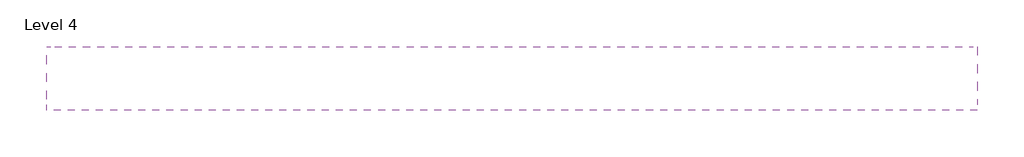
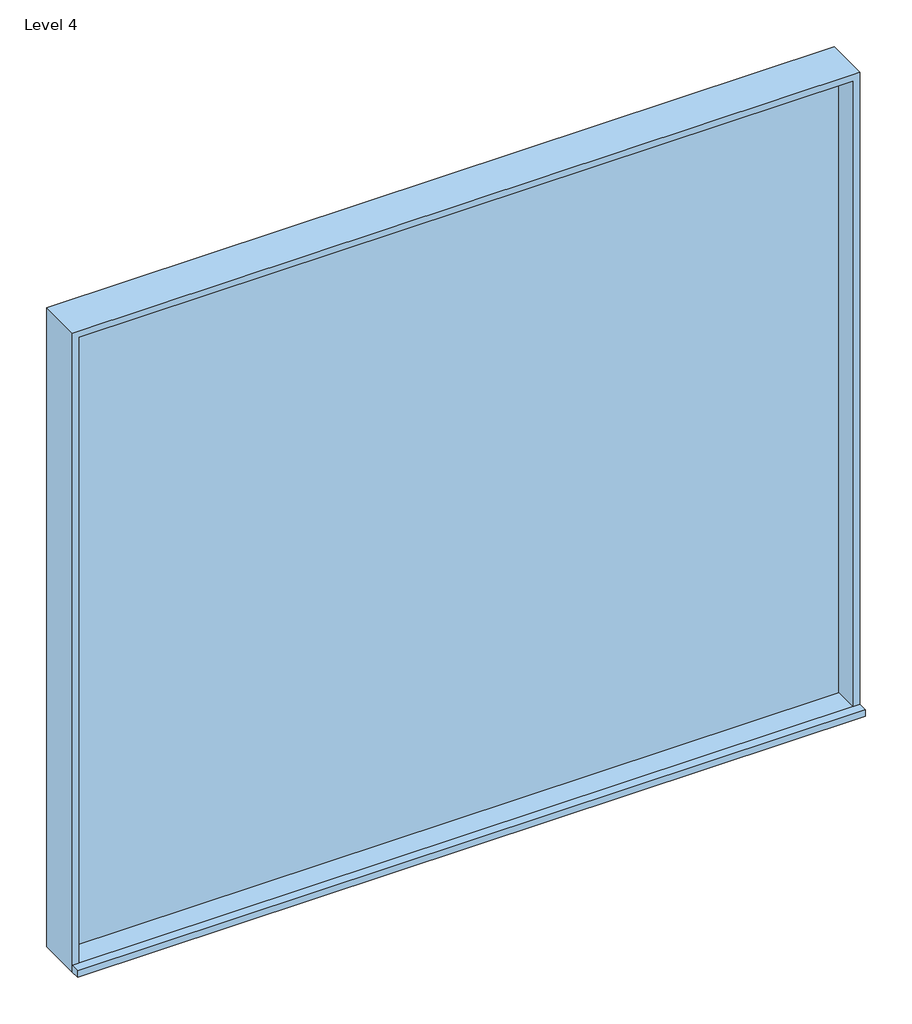
# One storey: 1 window.
"""IFC4 building model written with IfcOpenShell, lengths in millimetres."""

from ifc_helpers import new_model, si_unit, origin, place, context, project, spatial, transform, mapped, element, save
from components import window_88b07bfa

model = new_model("IFC4")

# Units and contexts
model_context = context("Model", 3, world=origin())
ifc_project = project(units=[si_unit("LENGTHUNIT", "METRE", prefix="MILLI")], contexts=[model_context])

# Site, building, storey
site = spatial("IfcSite", under=ifc_project)
building = spatial("IfcBuilding", under=site)
storey = spatial("IfcBuildingStorey", under=building, Name="Level 4", Elevation=9144.0)

# Window
placement = place(None, origin())
window_shape = window_88b07bfa(model_context)
element("IfcWindow", 1, ObjectType="Instance - Fixed : 24\" x 48\"", at=placement, inside=storey, context=model_context, shape_type="MappedRepresentation", body=[
    mapped(window_shape, transform((-10747.8874719, -885.9632813, 10301.8483945), x_axis=(-1.0, 0.0, 0.0), y_axis=(0.0, -1.0, 0.0), z_axis=(0.0, 0.0, 1.0))),
])

save(model, "model.ifc")

# Revit data of these elements
# Type "Instance - Fixed : 24\" x 48\""
#   Type Mark = "10"
#   Construction Type Id = "GSP4R"
#   Assembly Code = "B2020100"
#   Analytic Construction = "1/8 in Pilkington single glazing"
#   Visual Light Transmittance = 0.9
#   Thermal Resistance (R) = 0.8466 (h·ft²·°F)/BTU
#   Solar Heat Gain Coefficient = 0.86
#   Heat Transfer Coefficient (U) = 1.1812 BTU/(h·ft²·°F)
#   Height [instance default] = 4' - 0"
#   Default Sill Height = 3' - 0"
#   Width [instance default] = 2' - 0"
#   Window Inset = 0' - 2"
#   Define Thermal Properties by = 1
#   Glass Pane Material = Glass
#   Sash Material = Iron, Ductile
#   Wall Closure = (empty or 0)
# Element 1 (IfcWindow, "Instance - Fixed : 24\" x 48\"")
#   Mark = "4"
#   Width = 7' - 0"
#   Height = 6' - 0"
#   Phase Created = New Construction
#   Materials on its faces: "Iron, Ductile", "Glass"
# Materials
#   "Glass": class "Glass", colour RGB 0 128 192, transparency 0.75, Description = "Soda Lime Glass", Cost = 0
#   "Iron, Ductile": class "Metal", colour RGB 0 0 0, transparency 0, Description = "Ductile cast iron", Cost = 0
